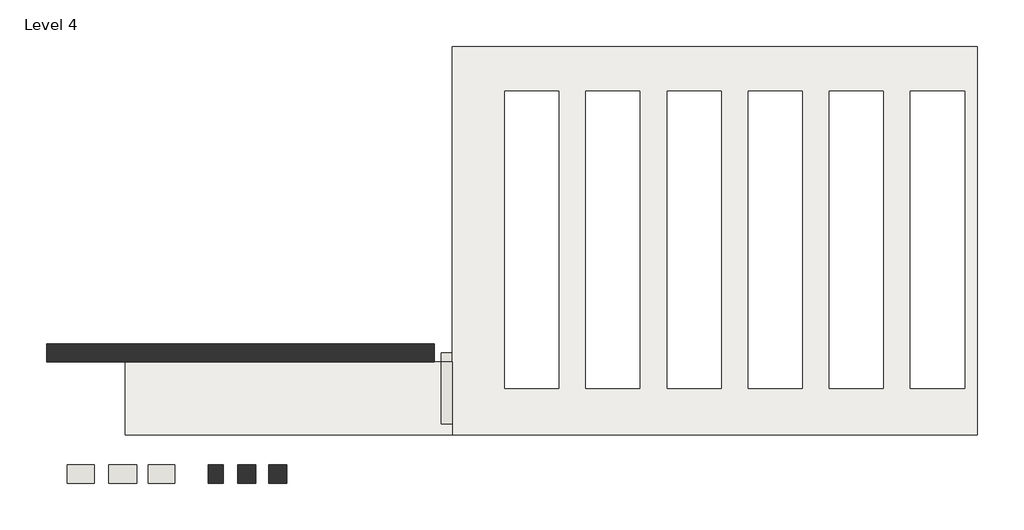
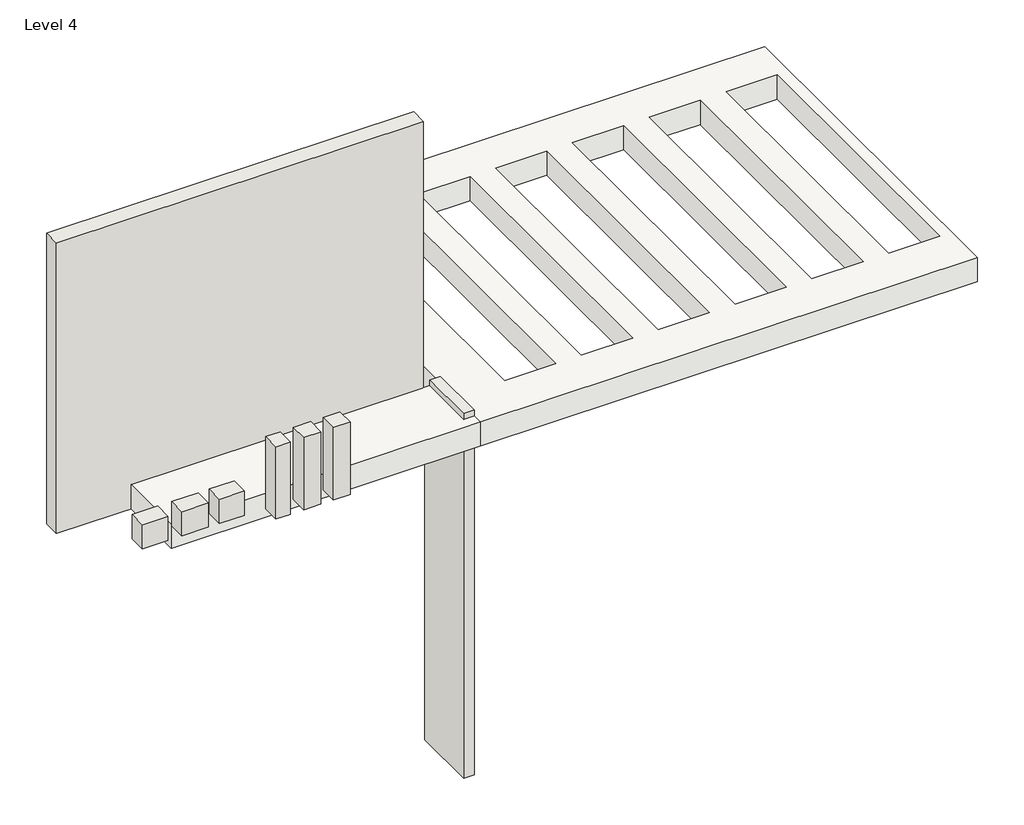
# One storey: 3 walls, 2 roofs.
"""IFC4 building model written with IfcOpenShell, lengths in millimetres."""

from ifc_helpers import new_model, si_unit, frame, origin, place, context, project, spatial, polyline, outline, extrude, faceted_brep, transform, mapped, element, save
from components import walls_4_walls_4_5f3310eb

model = new_model("IFC4")

# Units and contexts
model_context = context("Model", 3, world=origin())
ifc_project = project(units=[si_unit("LENGTHUNIT", "METRE", prefix="MILLI")], contexts=[model_context])

# Site, building, storey
site = spatial("IfcSite", under=ifc_project)
building = spatial("IfcBuilding", under=site)
storey = spatial("IfcBuildingStorey", under=building, Name="Level 4", Elevation=10972.8)

# Roofs
placement = place(None, origin())
element("IfcRoof", 1, ObjectType="Generic - 12\"", at=placement, inside=storey, context=model_context, shape_type="SweptSolid", body=[
    extrude(outline(polyline([(-7613.3936733, 4738.4419215), (-3930.3936733, 4738.4419215), (-3930.3936733, 3912.9419215), (-7613.3936733, 3912.9419215), (-7613.3936733, 4738.4419215)])), frame((0.0, 0.0, 10972.8), z_axis=(0.0, 0.0, 1.0), x_axis=(1.0, 0.0, 0.0)), (0.0, 0.0, 1.0), 304.8),
])
element("IfcRoof", 2, ObjectType="Generic - 12\"", at=placement, inside=storey, context=model_context, shape_type="SweptSolid", body=[
    extrude(outline(polyline([(-3930.3936733, 8294.4419215), (1986.1481409, 8294.4419215), (1986.1481409, 3912.9419215), (-3930.3936733, 3912.9419215), (-3930.3936733, 8294.4419215)]), holes=[polyline([(-2730.6760119, 4437.8066399), (-2730.6760119, 7790.6066399), (-3340.2760119, 7790.6066399), (-3340.2760119, 4437.8066399), (-2730.6760119, 4437.8066399)]), polyline([(-1816.2760119, 4437.8066399), (-1816.2760119, 7790.6066399), (-2425.8760119, 7790.6066399), (-2425.8760119, 4437.8066399), (-1816.2760119, 4437.8066399)]), polyline([(-901.8760119, 4437.8066399), (-901.8760119, 7790.6066399), (-1511.4760119, 7790.6066399), (-1511.4760119, 4437.8066399), (-901.8760119, 4437.8066399)]), polyline([(12.5239881, 4437.8066399), (12.5239881, 7790.6066399), (-597.0760119, 7790.6066399), (-597.0760119, 4437.8066399), (12.5239881, 4437.8066399)]), polyline([(926.9239881, 4437.8066399), (926.9239881, 7790.6066399), (317.3239881, 7790.6066399), (317.3239881, 4437.8066399), (926.9239881, 4437.8066399)]), polyline([(1841.3239881, 4437.8066399), (1841.3239881, 7790.6066399), (1231.7239881, 7790.6066399), (1231.7239881, 4437.8066399), (1841.3239881, 4437.8066399)])]), frame((0.0, 0.0, 10972.8), z_axis=(0.0, 0.0, 1.0), x_axis=(1.0, 0.0, 0.0)), (0.0, 0.0, 1.0), 304.8),
])

# Walls
element("IfcWall", 3, ObjectType="Generic - 5\"", at=placement, inside=storey, context=model_context, shape_type="Brep", body=[
    faceted_brep([(-4057.3936733, 4840.0419215, 6756.4), (-4057.3936733, 4039.9419215, 6756.4), (-4057.3936733, 4039.9419215, 11349.3315531), (-4057.3936733, 4738.4419215, 11349.3315531), (-4057.3936733, 4738.4419215, 10972.8), (-4057.3936733, 4840.0419215, 10972.8), (-3930.3936733, 4840.0419215, 6756.4), (-3930.3936733, 4840.0419215, 7315.2), (-3930.3936733, 4840.0419215, 10972.8), (-3930.3936733, 4738.4419215, 10972.8), (-3930.3936733, 4738.4419215, 11349.3315531), (-3930.3936733, 4039.9419215, 11349.3315531), (-3930.3936733, 4039.9419215, 11201.4), (-3930.3936733, 4039.9419215, 6756.4)], [[[0, 1, 2, 3, 4, 5]], [[6, 7, 8, 9, 10, 11, 12, 13]], [[1, 0, 6, 13]], [[3, 2, 11, 10]], [[0, 5, 8, 7, 6]], [[4, 9, 8, 5]], [[4, 3, 10, 9]], [[1, 13, 12, 11, 2]]]),
])
element("IfcWall", 4, ObjectType="Generic - 8\"", at=placement, inside=storey, context=model_context, shape_type="Brep", body=[
    faceted_brep([(-8502.3936733, 4738.4419215, 10972.8), (-7486.3936733, 4738.4419215, 10972.8), (-4133.5936733, 4738.4419215, 10972.8), (-4133.5936733, 4738.4419215, 14630.4), (-8502.3936733, 4738.4419215, 14630.4), (-8502.3936733, 4941.6419215, 10972.8), (-8502.3936733, 4941.6419215, 14630.4), (-4133.5936733, 4941.6419215, 14630.4), (-4133.5936733, 4941.6419215, 10972.8), (-8502.3936733, 4865.4419215, 10972.8), (-4133.5936733, 4840.0419215, 10972.8)], [[[0, 1, 2, 3, 4]], [[5, 6, 7, 8]], [[2, 1, 0, 9, 5, 8, 10]], [[4, 3, 7, 6]], [[0, 4, 6, 5, 9]], [[2, 10, 8, 7, 3]]]),
])
walls_4_walls_4_shape = walls_4_walls_4_5f3310eb(model_context)
element("IfcWall", 5, ObjectType="Walls 4 : Walls 4", at=placement, inside=storey, context=model_context, shape_type="MappedRepresentation", body=[
    mapped(walls_4_walls_4_shape, transform((0.0, 0.0, 0.0), x_axis=(1.0, 0.0, 0.0), y_axis=(0.0, 1.0, 0.0), z_axis=(0.0, 0.0, 1.0))),
])

save(model, "model.ifc")

# Revit data of these elements
# Type "Generic - 12\""
#   Assembly Code = "B1020"
#   Layers, outside or top first: 1' - 0" no material (function 1)
# Type "Generic - 5\""
#   Assembly Code = "B2010"
#   Layers, outside or top first: 0' - 5" no material (function 1)
# Type "Generic - 8\""
#   Assembly Code = "B2010"
#   Layers, outside or top first: 0' - 8" no material (function 1)
# Elements 1, 2 (IfcRoof, "Generic - 12\"")
#   built-in parameter 1001705 = 37 (stored number, unit not read)
#   built-in parameter 1001710 = 33615
#   Phase Created = New Construction
#   Materials on its faces: "Default Roof"
# Element 3 (IfcWall, "Generic - 5\"")
#   built-in parameter 1001111 = -13' - 10"
#   Top Offset = -10' - 9.17592"
#   Base Offset = -13' - 10"
#   wall height = 15' - 0.82408"
#   Phase Created = New Construction
#   Base Constraint = Level 4
#   Top Constraint = Level 5
#   Materials on its faces: "Default Wall"
# Element 4 (IfcWall, "Generic - 8\"")
#   Top Offset = 0' - 0"
#   Base Offset = 0' - 0"
#   Unconnected Height = 12' - 0"
#   wall height = 12' - 0"
#   Phase Created = New Construction
#   Base Constraint = Level 4
#   Materials on its faces: "Default Wall"
# Element 5 (IfcWall, "Walls 4 : Walls 4")
#   Phase Created = New Construction
#   Materials on its faces: "Default Wall"
# Materials
#   "Default Roof": colour RGB 88 101 114, transparency 0
#   "Default Wall": colour RGB 128 128 128, transparency 0
